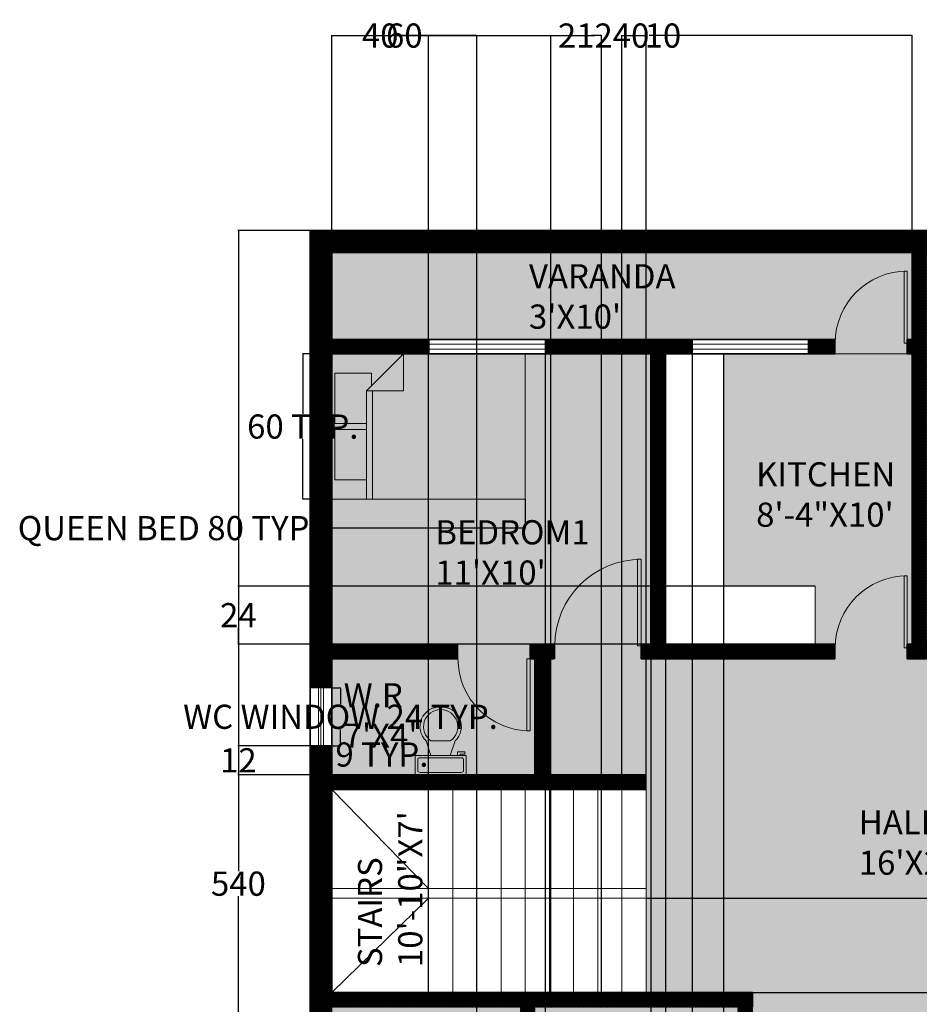
# Model space of a CAD drawing. Units: inches. Extents: x -89252 to 1164, y -183799 to 823.
# Tile 3 of 4: x 600 to 972, y 416 to 823. Entities that reach past the tile are written whole.
import ezdxf

# ---------------------------------------------------------------- set-up
doc = ezdxf.new("R2010")
doc.units = ezdxf.units.IN
doc.header["$MEASUREMENT"] = 0
for name, color, linetype, lineweight in [('A-ANNO-DIMS', 2, 'Continuous', 18), ('A-AREA-IDEN', 7, 'Continuous', 25), ('A-FLOR-CASE', 8, 'Continuous', 18), ('A-FLOR-STRS', 7, 'Continuous', 18), ('A-GLAZ', 4, 'Continuous', 18), ('A-WALL', 7, 'Continuous', 35), ('BED', 7, 'Continuous', 18), ('DOOR', 7, 'Continuous', 18), ('TOILET', 7, 'Continuous', 18)]:
    doc.layers.add(name, color=color, linetype=linetype, lineweight=lineweight)
doc.layers.add('A-FLOR-PATT', color=252, linetype='Continuous', lineweight=13, true_color=0x939598)
doc.layers.add('A-WALL-PATT', color=18, linetype='Continuous', lineweight=13, true_color=0x000000)
doc.styles.get("Standard").update_dxf_attribs({"font": 'arial.ttf'})
doc.dimstyles.get("Standard").update_dxf_attribs({"dimtxt": 10, "dimasz": 0.18, "dimexe": 0.18, "dimexo": 0.0625, "dimgap": 0.09, "dimtad": 0, "dimtih": 1, "dimtoh": 1, "dimdec": 0, "dimzin": 0, "dimdsep": 46, "dimlunit": 3, "dimtxsty": 'Standard', "dimcen": 0.09, "dimadec": 0, "dimazin": 0, "dimtfac": 1, "dimtdec": 0, "dimtofl": 0, "dimtmove": 0, "dimatfit": 3, "dimfxl": 1, "dimtolj": 1, "dimtzin": 0, "dimarcsym": 0})

# ---------------------------------------------------------------- blocks, each defined once
blk = doc.blocks.new('*U3')
for p, q in [((0, 0), (0, -6)), ((40, 0), (40, -6))]:
    blk.add_line(p, q)
blk.add_lwpolyline([(0, 0), (0, 40), (1.75, 40), (1.75, 0)], close=True)
blk.add_arc((0, 0), 40, 0, 90)
blk = doc.blocks.new('*U4')
for p, q in [((0, 0), (0, 6)), ((40, 0), (40, 6))]:
    blk.add_line(p, q)
blk.add_lwpolyline([(0, 0), (0, -40), (1.75, -40), (1.75, 0)], close=True)
blk.add_arc((0, 0), 40, 270, 0)
blk = doc.blocks.new('Bed - Queen')
for p, q in [((0, -80.00003), (0, 0)), ((0, 0), (59.99999, 0)), ((59.99999, 0), (59.99999, -80.00003)), ((7.99999, -1.2), (28.79998, -1.2)), ((7.99999, -14.4), (7.99999, -1.2)), ((28.79998, -1.2), (28.79998, -14.4)), ((31.19999, -1.2), (51.99999, -1.2)), ((31.19999, -14.4), (31.19999, -1.2)), ((51.99999, -1.2), (51.99999, -16.4)), ((0, -14.4), (44.8, -14.4)), ((59.99999, -29.6), (44.8, -14.4)), ((44.8, -14.4), (44.8, -29.6)), ((44.8, -16.8), (0, -16.8)), ((51.99999, -16.4), (46.79936, -16.4)), ((44.8, -29.6), (59.99999, -29.6)), ((59.99999, -80.00003), (0, -80.00003))]:
    blk.add_line(p, q)
blk = doc.blocks.new('*U12')
for p, q in [((9.5, -6), (9.5, -2)), ((-8, -8.5), (-8, -8)), ((-7, -8), (-7, -9.5)), ((-4, -8), (-6, -14)), ((4, -8), (6, -14)), ((-10, -8.5), (-8, -8.5)), ((-10, -9.5), (-10, -8.5)), ((-7, -9.5), (-10, -9.5)), ((4, -14), (-4, -14))]:
    blk.add_line(p, q)
blk.add_lwpolyline([(10.5, -8), (10.5, 0), (-10.5, 0), (-10.5, -8)], close=True)
for points in [[(-9.5, -2), (-9.5, -6)], [(8.5, -1), (-8.5, -1)], [(-8.5, -7), (8.5, -7)]]:
    blk.add_lwpolyline(points)
for centre, radius, start, end in [((-8.625, -1.875), 0.8839, 81.8699, 188.1301), ((8.625, -1.875), 0.8839, 351.8699, 98.1301), ((-8.625, -6.125), 0.8839, 171.869898, 278.1301), ((8.625, -6.125), 0.8839, 261.8699, 8.1301), ((-0.4772, -19.9188), 8.0953, 133.01722, 273.38), ((0.0374, -19.8731), 7.127, 124.50543, 269.7), ((-0.0373, -19.8731), 7.127, 270.3, 55.4946), ((0.4773, -19.9188), 8.0953, 266.62, 46.9828)]:
    blk.add_arc(centre, radius, start, end)
blk = doc.blocks.new('WIN-24IN-9IN-WALL')
for p, q in [((9, 24), (0, 24)), ((3.5, 0), (3.5, 24)), ((4.5, 0), (4.5, 24)), ((5.5, 0), (5.5, 24)), ((9, 0), (0, 0))]:
    blk.add_line(p, q)
blk = doc.blocks.new('WIN-48IN-6IN-WALL')
for p, q in [((0, 0), (0, 6)), ((48, 0), (48, 6)), ((0, 4), (48, 4)), ((0, 2), (48, 2))]:
    blk.add_line(p, q)
blk = doc.blocks.new('*D18')
at = {"layer": 'A-ANNO-DIMS', "color": 0, "lineweight": -2, "transparency": 16777216}
for p, q in [((729.36, 624.33), (729.36, 612.21)), ((809.36, 624.33), (809.36, 612.21)), ((729.36, 612.39), (729.18, 612.39)), ((809.18, 612.39), (729.54, 612.39))]:
    blk.add_line(p, q, dxfattribs=at)
at = {"layer": 'A-ANNO-DIMS', "color": 0, "transparency": 16777216}
for points in [[(729.54, 612.42), (729.54, 612.36), (729.36, 612.39)], [(809.18, 612.42), (809.18, 612.36), (809.36, 612.39)]]:
    blk.add_solid(points, dxfattribs=at)
at = {"layer": 'Defpoints', "color": 0, "transparency": 16777216}
for p in [(729.36, 624.39), (809.36, 624.39), (729.36, 612.39)]:
    blk.add_point(p, dxfattribs=at)
at = {"layer": 'A-ANNO-DIMS', "color": 0, "transparency": 16777216, "insert": (661.68, 612.39), "char_height": 10, "attachment_point": 5}
blk.add_mtext('\\A1;QUEEN BED 80 TYP.', dxfattribs=at)
blk = doc.blocks.new('*D19')
at = {"layer": 'A-ANNO-DIMS', "color": 0, "lineweight": -2, "transparency": 16777216}
for p, q in [((729.3, 684.39), (717.18, 684.39)), ((717.36, 684.21), (717.36, 659.59)), ((717.36, 624.57), (717.36, 649.19)), ((729.3, 624.39), (717.18, 624.39))]:
    blk.add_line(p, q, dxfattribs=at)
at = {"layer": 'A-ANNO-DIMS', "color": 0, "transparency": 16777216}
for points in [[(717.33, 684.21), (717.39, 684.21), (717.36, 684.39)], [(717.33, 624.57), (717.39, 624.57), (717.36, 624.39)]]:
    blk.add_solid(points, dxfattribs=at)
at = {"layer": 'Defpoints', "color": 0, "transparency": 16777216}
for p in [(717.36, 684.39), (729.36, 684.39), (729.36, 624.39)]:
    blk.add_point(p, dxfattribs=at)
at = {"layer": 'A-ANNO-DIMS', "color": 0, "transparency": 16777216, "insert": (717.36, 654.39), "char_height": 10, "attachment_point": 5}
blk.add_mtext('\\A1;60 TYP.', dxfattribs=at)
blk = doc.blocks.new('*D20')
at = {"layer": 'A-ANNO-DIMS', "color": 0, "lineweight": -2, "transparency": 16777216}
for p, q in [((729.43, 546.39), (733.14, 546.39)), ((732.96, 546.21), (732.96, 539.65)), ((732.96, 522.57), (732.96, 529.13)), ((729.43, 522.39), (733.14, 522.39))]:
    blk.add_line(p, q, dxfattribs=at)
at = {"layer": 'A-ANNO-DIMS', "color": 0, "transparency": 16777216}
for points in [[(732.93, 546.21), (732.99, 546.21), (732.96, 546.39)], [(732.93, 522.57), (732.99, 522.57), (732.96, 522.39)]]:
    blk.add_solid(points, dxfattribs=at)
at = {"layer": 'Defpoints', "color": 0, "transparency": 16777216}
for p in [(729.36, 546.39), (732.96, 546.39), (729.36, 522.39)]:
    blk.add_point(p, dxfattribs=at)
at = {"layer": 'A-ANNO-DIMS', "color": 0, "transparency": 16777216, "insert": (732.96, 534.39), "char_height": 10, "attachment_point": 5}
blk.add_mtext('\\A1;WC WINDOW 24 TYP.', dxfattribs=at)
blk = doc.blocks.new('*D21')
at = {"layer": 'A-ANNO-DIMS', "color": 0, "lineweight": -2, "transparency": 16777216}
for p, q in [((720.36, 522.33), (720.36, 518.61)), ((729.36, 522.33), (729.36, 518.61)), ((720.54, 518.79), (729.18, 518.79)), ((729.36, 518.79), (729.54, 518.79))]:
    blk.add_line(p, q, dxfattribs=at)
at = {"layer": 'A-ANNO-DIMS', "color": 0, "transparency": 16777216}
for points in [[(720.54, 518.82), (720.54, 518.76), (720.36, 518.79)], [(729.18, 518.82), (729.18, 518.76), (729.36, 518.79)]]:
    blk.add_solid(points, dxfattribs=at)
at = {"layer": 'Defpoints', "color": 0, "transparency": 16777216}
for p in [(720.36, 522.39), (729.36, 522.39), (729.36, 518.79)]:
    blk.add_point(p, dxfattribs=at)
at = {"layer": 'A-ANNO-DIMS', "color": 0, "transparency": 16777216, "insert": (750.09, 518.79), "char_height": 10, "attachment_point": 5}
blk.add_mtext('\\A1;9 TYP.', dxfattribs=at)
blk = doc.blocks.new('*D31')
at = {"layer": 'A-ANNO-DIMS', "color": 0, "lineweight": -2, "transparency": 16777216}
for p, q in [((720.3, 735.39), (690.53, 735.39)), ((690.71, 735.21), (690.71, 470.59)), ((690.71, 195.57), (690.71, 460.19)), ((720.3, 195.39), (690.53, 195.39))]:
    blk.add_line(p, q, dxfattribs=at)
at = {"layer": 'A-ANNO-DIMS', "color": 0, "transparency": 16777216}
for points in [[(690.68, 735.21), (690.74, 735.21), (690.71, 735.39)], [(690.68, 195.57), (690.74, 195.57), (690.71, 195.39)]]:
    blk.add_solid(points, dxfattribs=at)
at = {"layer": 'Defpoints', "color": 0, "transparency": 16777216}
for p in [(690.71, 735.39), (720.36, 735.39), (720.36, 195.39)]:
    blk.add_point(p, dxfattribs=at)
at = {"layer": 'A-ANNO-DIMS', "color": 0, "transparency": 16777216, "insert": (690.71, 465.39), "char_height": 10, "attachment_point": 5}
blk.add_mtext('\\A1;540', dxfattribs=at)
blk = doc.blocks.new('*D33')
at = {"layer": 'A-ANNO-DIMS', "color": 0, "lineweight": -2, "transparency": 16777216}
for p, q in [((729.36, 726.45), (729.36, 816.22)), ((729.54, 816.04), (838.16, 816.04)), ((969.18, 816.04), (860.57, 816.04)), ((969.36, 726.45), (969.36, 816.22))]:
    blk.add_line(p, q, dxfattribs=at)
at = {"layer": 'A-ANNO-DIMS', "color": 0, "transparency": 16777216}
for points in [[(729.54, 816.07), (729.54, 816.01), (729.36, 816.04)], [(969.18, 816.07), (969.18, 816.01), (969.36, 816.04)]]:
    blk.add_solid(points, dxfattribs=at)
at = {"layer": 'Defpoints', "color": 0, "transparency": 16777216}
for p in [(969.36, 816.04), (729.36, 726.39), (969.36, 726.39)]:
    blk.add_point(p, dxfattribs=at)
at = {"layer": 'A-ANNO-DIMS', "color": 0, "transparency": 16777216, "insert": (849.36, 816.04), "char_height": 10, "attachment_point": 5}
blk.add_mtext('\\A1;240', dxfattribs=at)
blk = doc.blocks.new('*D41')
at = {"layer": 'A-ANNO-DIMS', "color": 0, "lineweight": -2, "transparency": 16777216}
for p, q in [((729.36, 240.45), (729.36, 816.22)), ((729.54, 816.04), (752.1, 816.04)), ((789.18, 816.04), (766.63, 816.04)), ((789.36, 240.45), (789.36, 816.22))]:
    blk.add_line(p, q, dxfattribs=at)
at = {"layer": 'A-ANNO-DIMS', "color": 0, "transparency": 16777216}
for points in [[(729.54, 816.07), (729.54, 816.01), (729.36, 816.04)], [(789.18, 816.07), (789.18, 816.01), (789.36, 816.04)]]:
    blk.add_solid(points, dxfattribs=at)
at = {"layer": 'Defpoints', "color": 0, "transparency": 16777216}
for p in [(789.36, 816.04), (729.36, 240.39), (789.36, 240.39)]:
    blk.add_point(p, dxfattribs=at)
at = {"layer": 'A-ANNO-DIMS', "color": 0, "transparency": 16777216, "insert": (759.36, 816.04), "char_height": 10, "attachment_point": 5}
blk.add_mtext('\\A1;60', dxfattribs=at)
blk = doc.blocks.new('*D43')
at = {"layer": 'A-ANNO-DIMS', "color": 0, "lineweight": -2, "transparency": 16777216}
for p, q in [((849.36, 504.45), (849.36, 816.22)), ((849.54, 816.04), (859.18, 816.04)), ((859.36, 504.45), (859.36, 816.22)), ((859.36, 816.04), (859.54, 816.04))]:
    blk.add_line(p, q, dxfattribs=at)
at = {"layer": 'A-ANNO-DIMS', "color": 0, "transparency": 16777216}
for points in [[(849.54, 816.07), (849.54, 816.01), (849.36, 816.04)], [(859.18, 816.07), (859.18, 816.01), (859.36, 816.04)]]:
    blk.add_solid(points, dxfattribs=at)
at = {"layer": 'Defpoints', "color": 0, "transparency": 16777216}
for p in [(859.36, 816.04), (849.36, 504.39), (859.36, 504.39)]:
    blk.add_point(p, dxfattribs=at)
at = {"layer": 'A-ANNO-DIMS', "color": 0, "transparency": 16777216, "insert": (866.31, 816.04), "char_height": 10, "attachment_point": 5}
blk.add_mtext('\\A1;10', dxfattribs=at)
blk = doc.blocks.new('*D44')
at = {"layer": 'A-ANNO-DIMS', "color": 0, "lineweight": -2, "transparency": 16777216}
for p, q in [((867.36, 684.33), (867.36, 165.56)), ((891.36, 684.33), (891.36, 165.56)), ((867.54, 165.74), (872.05, 165.74)), ((891.18, 165.74), (886.68, 165.74))]:
    blk.add_line(p, q, dxfattribs=at)
at = {"layer": 'A-ANNO-DIMS', "color": 0, "transparency": 16777216}
for points in [[(867.54, 165.77), (867.54, 165.71), (867.36, 165.74)], [(891.18, 165.77), (891.18, 165.71), (891.36, 165.74)]]:
    blk.add_solid(points, dxfattribs=at)
at = {"layer": 'Defpoints', "color": 0, "transparency": 16777216}
for p in [(867.36, 684.39), (891.36, 684.39), (891.36, 165.74)]:
    blk.add_point(p, dxfattribs=at)
at = {"layer": 'A-ANNO-DIMS', "color": 0, "transparency": 16777216, "insert": (879.36, 165.74), "char_height": 10, "attachment_point": 5}
blk.add_mtext('\\A1;24', dxfattribs=at)
blk = doc.blocks.new('*D45')
at = {"layer": 'A-ANNO-DIMS', "color": 0, "lineweight": -2, "transparency": 16777216}
for p, q in [((929.24, 588.39), (690.53, 588.39)), ((690.71, 588.21), (690.71, 581.5)), ((690.71, 564.57), (690.71, 571.28)), ((929.24, 564.39), (690.53, 564.39))]:
    blk.add_line(p, q, dxfattribs=at)
at = {"layer": 'A-ANNO-DIMS', "color": 0, "transparency": 16777216}
for points in [[(690.68, 588.21), (690.74, 588.21), (690.71, 588.39)], [(690.68, 564.57), (690.74, 564.57), (690.71, 564.39)]]:
    blk.add_solid(points, dxfattribs=at)
at = {"layer": 'Defpoints', "color": 0, "transparency": 16777216}
for p in [(690.71, 588.39), (929.31, 588.39), (929.31, 564.39)]:
    blk.add_point(p, dxfattribs=at)
at = {"layer": 'A-ANNO-DIMS', "color": 0, "transparency": 16777216, "insert": (690.71, 576.39), "char_height": 10, "attachment_point": 5}
blk.add_mtext('\\A1;24', dxfattribs=at)
blk = doc.blocks.new('*D47')
at = {"layer": 'A-ANNO-DIMS', "color": 0, "lineweight": -2, "transparency": 16777216}
for p, q in [((817.67, 690.33), (817.67, 165.56)), ((878.36, 690.33), (878.36, 165.56)), ((817.85, 165.74), (831.02, 165.74)), ((878.18, 165.74), (865.02, 165.74))]:
    blk.add_line(p, q, dxfattribs=at)
at = {"layer": 'A-ANNO-DIMS', "color": 0, "transparency": 16777216}
for points in [[(817.85, 165.77), (817.85, 165.71), (817.67, 165.74)], [(878.18, 165.77), (878.18, 165.71), (878.36, 165.74)]]:
    blk.add_solid(points, dxfattribs=at)
at = {"layer": 'Defpoints', "color": 0, "transparency": 16777216}
for p in [(817.67, 690.39), (878.36, 690.39), (878.36, 165.74)]:
    blk.add_point(p, dxfattribs=at)
at = {"layer": 'A-ANNO-DIMS', "color": 0, "transparency": 16777216, "insert": (848.02, 165.74), "char_height": 10, "attachment_point": 5}
blk.add_mtext('\\A1;60.69', dxfattribs=at)
blk = doc.blocks.new('*D48')
at = {"layer": 'A-ANNO-DIMS', "color": 0, "lineweight": -2, "transparency": 16777216}
for p, q in [((817.67, 684.33), (817.67, 165.56)), ((861.36, 684.33), (861.36, 165.56)), ((817.85, 165.74), (822.34, 165.74)), ((861.18, 165.74), (856.69, 165.74))]:
    blk.add_line(p, q, dxfattribs=at)
at = {"layer": 'A-ANNO-DIMS', "color": 0, "transparency": 16777216}
for points in [[(817.85, 165.77), (817.85, 165.71), (817.67, 165.74)], [(861.18, 165.77), (861.18, 165.71), (861.36, 165.74)]]:
    blk.add_solid(points, dxfattribs=at)
at = {"layer": 'Defpoints', "color": 0, "transparency": 16777216}
for p in [(817.67, 684.39), (861.36, 684.39), (861.36, 165.74)]:
    blk.add_point(p, dxfattribs=at)
at = {"layer": 'A-ANNO-DIMS', "color": 0, "transparency": 16777216, "insert": (839.52, 165.74), "char_height": 10, "attachment_point": 5}
blk.add_mtext('\\A1;43.69', dxfattribs=at)
blk = doc.blocks.new('*D50')
at = {"layer": 'A-ANNO-DIMS', "color": 0, "lineweight": -2, "transparency": 16777216}
for p, q in [((729.3, 522.39), (690.53, 522.39)), ((690.71, 522.21), (690.71, 521.5)), ((729.3, 510.39), (690.53, 510.39)), ((690.71, 510.57), (690.71, 511.28))]:
    blk.add_line(p, q, dxfattribs=at)
at = {"layer": 'A-ANNO-DIMS', "color": 0, "transparency": 16777216}
for points in [[(690.68, 522.21), (690.74, 522.21), (690.71, 522.39)], [(690.68, 510.57), (690.74, 510.57), (690.71, 510.39)]]:
    blk.add_solid(points, dxfattribs=at)
at = {"layer": 'Defpoints', "color": 0, "transparency": 16777216}
for p in [(729.36, 522.39), (690.71, 510.39), (729.36, 510.39)]:
    blk.add_point(p, dxfattribs=at)
at = {"layer": 'A-ANNO-DIMS', "color": 0, "transparency": 16777216, "insert": (690.71, 516.39), "char_height": 10, "attachment_point": 5}
blk.add_mtext('\\A1;12', dxfattribs=at)
blk = doc.blocks.new('*D51')
at = {"layer": 'A-ANNO-DIMS', "color": 0, "lineweight": -2, "transparency": 16777216}
for p, q in [((729.36, 420.45), (729.36, 816.22)), ((729.54, 816.04), (741.93, 816.04)), ((769.18, 816.04), (756.8, 816.04)), ((769.36, 420.45), (769.36, 816.22))]:
    blk.add_line(p, q, dxfattribs=at)
at = {"layer": 'A-ANNO-DIMS', "color": 0, "transparency": 16777216}
for points in [[(729.54, 816.07), (729.54, 816.01), (729.36, 816.04)], [(769.18, 816.07), (769.18, 816.01), (769.36, 816.04)]]:
    blk.add_solid(points, dxfattribs=at)
at = {"layer": 'Defpoints', "color": 0, "transparency": 16777216}
for p in [(729.36, 816.04), (729.36, 420.39), (769.36, 420.39)]:
    blk.add_point(p, dxfattribs=at)
at = {"layer": 'A-ANNO-DIMS', "color": 0, "transparency": 16777216, "insert": (749.36, 816.04), "char_height": 10, "attachment_point": 5}
blk.add_mtext('\\A1;40', dxfattribs=at)
blk = doc.blocks.new('*D52')
at = {"layer": 'A-ANNO-DIMS', "color": 0, "lineweight": -2, "transparency": 16777216}
for p, q in [((859.43, 459.39), (1134.19, 459.39)), ((1134.01, 459.21), (1134.01, 445.09)), ((1134.01, 420.57), (1134.01, 434.69)), ((859.43, 420.39), (1134.19, 420.39))]:
    blk.add_line(p, q, dxfattribs=at)
at = {"layer": 'A-ANNO-DIMS', "color": 0, "transparency": 16777216}
for points in [[(1133.98, 459.21), (1134.04, 459.21), (1134.01, 459.39)], [(1133.98, 420.57), (1134.04, 420.57), (1134.01, 420.39)]]:
    blk.add_solid(points, dxfattribs=at)
at = {"layer": 'Defpoints', "color": 0, "transparency": 16777216}
for p in [(859.36, 459.39), (1134.01, 459.39), (859.36, 420.39)]:
    blk.add_point(p, dxfattribs=at)
at = {"layer": 'A-ANNO-DIMS', "color": 0, "transparency": 16777216, "insert": (1134.01, 439.89), "char_height": 10, "attachment_point": 5}
blk.add_mtext('\\A1;39', dxfattribs=at)
blk = doc.blocks.new('*D53')
at = {"layer": 'A-ANNO-DIMS', "color": 0, "lineweight": -2, "transparency": 16777216}
for p, q in [((819.96, 414.26), (819.96, 816.22)), ((820.14, 816.04), (824.09, 816.04)), ((840.78, 816.04), (836.83, 816.04)), ((840.96, 414.26), (840.96, 816.22))]:
    blk.add_line(p, q, dxfattribs=at)
at = {"layer": 'A-ANNO-DIMS', "color": 0, "transparency": 16777216}
for points in [[(820.14, 816.07), (820.14, 816.01), (819.96, 816.04)], [(840.78, 816.07), (840.78, 816.01), (840.96, 816.04)]]:
    blk.add_solid(points, dxfattribs=at)
at = {"layer": 'Defpoints', "color": 0, "transparency": 16777216}
for p in [(840.96, 816.04), (819.96, 414.2), (840.96, 414.2)]:
    blk.add_point(p, dxfattribs=at)
at = {"layer": 'A-ANNO-DIMS', "color": 0, "transparency": 16777216, "insert": (830.46, 816.04), "char_height": 10, "attachment_point": 5}
blk.add_mtext('\\A1;21', dxfattribs=at)

msp = doc.modelspace()

# ---------------------------------------------------------------- hatches: boundary and pattern name
at = {"layer": 'A-FLOR-PATT'}
h = msp.add_hatch(color=256, dxfattribs=at)
h.dxf.hatch_style = 1
h.paths.add_polyline_path([(1095.364, 558.3893), (1013.364, 558.3893), (1013.364, 564.3893), (1095.364, 564.3893), (1095.364, 672.3893), (1093.364, 672.3893), (1063.364, 672.3893), (1005.364, 672.3893), (1005.364, 726.3893), (975.364, 726.3893), (975.364, 690.3893), (975.364, 564.3893), (977.364, 564.3893), (977.364, 558.3893), (975.364, 558.3893), (969.364, 558.3893), (967.364, 558.3893), (967.364, 564.3893), (969.364, 564.3893), (969.364, 684.3893), (967.364, 684.3893), (937.364, 684.3893), (891.364, 684.3893), (891.364, 588.3893), (929.3053, 588.3893), (929.3053, 564.3893), (937.364, 564.3893), (937.364, 558.3893), (857.364, 558.3893), (857.364, 564.3893), (861.364, 564.3893), (861.364, 684.3893), (729.364, 684.3893), (729.364, 564.3893), (781.364, 564.3893), (781.364, 558.3893), (729.364, 558.3893), (729.364, 510.3893), (813.364, 510.3893), (813.364, 558.3893), (811.364, 558.3893), (811.364, 564.3893), (813.364, 564.3893), (819.364, 564.3893), (821.364, 564.3893), (821.364, 558.3893), (819.364, 558.3893), (819.364, 510.3893), (859.364, 510.3893), (859.364, 420.3893), (903.364, 420.3893), (903.364, 414.3893), (903.364, 412.3893), (897.364, 412.3893), (897.364, 414.3893), (813.364, 414.3893), (813.364, 366.3893), (897.364, 366.3893), (897.364, 382.3893), (903.364, 382.3893), (903.364, 360.3893), (903.364, 358.3893), (897.364, 358.3893), (897.364, 360.3893), (807.364, 360.3893), (805.364, 360.3893), (805.364, 366.3893), (807.364, 366.3893), (807.364, 414.3893), (729.364, 414.3893), (729.364, 366.3893), (775.364, 366.3893), (775.364, 360.3893), (729.364, 360.3893), (729.364, 240.3893), (897.364, 240.3893), (897.364, 318.3893), (1021.364, 318.3893), (1021.364, 312.3893), (1071.364, 312.3893), (1071.364, 318.3893), (1095.364, 318.3893)])
h.paths.add_polyline_path([(1095.364, 726.3893), (1011.364, 726.3893), (1011.364, 678.3893), (1063.364, 678.3893), (1063.364, 672.3893), (1093.364, 672.3893), (1093.364, 678.3893), (1095.364, 678.3893)])
h.paths.add_polyline_path([(969.364, 726.3893), (729.364, 726.3893), (729.364, 690.3893), (937.364, 690.3893), (937.364, 684.3893), (967.364, 684.3893), (967.364, 690.3893), (969.364, 690.3893)])
at = {"layer": 'A-WALL-PATT'}
h = msp.add_hatch(dxfattribs=at)
h.set_pattern_fill('ANSI31', color=256)
h.paths.add_polyline_path([(867.364, 684.3893), (878.364, 684.3893), (878.364, 690.3893), (817.6735, 690.3893), (817.6735, 684.3893), (861.364, 684.3893), (861.364, 564.3893), (857.364, 564.3893), (857.364, 558.3893), (937.364, 558.3893), (937.364, 564.3893), (867.364, 564.3893)], flags=17)
h.paths.add_polyline_path([(1041.364, 735.3893), (720.364, 735.3893), (720.364, 546.3893), (729.364, 546.3893), (729.364, 558.3893), (781.364, 558.3893), (781.364, 564.3893), (729.364, 564.3893), (729.364, 684.3893), (769.6735, 684.3893), (769.6735, 690.3893), (729.364, 690.3893), (729.364, 726.3893), (969.364, 726.3893), (969.364, 690.3893), (967.364, 690.3893), (967.364, 684.3893), (969.364, 684.3893), (969.364, 564.3893), (967.364, 564.3893), (967.364, 558.3893), (969.364, 558.3893), (975.364, 558.3893), (977.364, 558.3893), (977.364, 564.3893), (975.364, 564.3893), (975.364, 690.3893), (975.364, 726.3893), (1005.364, 726.3893), (1005.364, 672.3893), (1063.364, 672.3893), (1063.364, 678.3893), (1011.364, 678.3893), (1011.364, 726.3893), (1041.364, 726.3893)])
h.paths.add_polyline_path([(1104.364, 735.3893), (1065.364, 735.3893), (1065.364, 726.3893), (1095.364, 726.3893), (1095.364, 678.3893), (1093.364, 678.3893), (1093.364, 672.3893), (1095.364, 672.3893), (1095.364, 642.3893), (1104.364, 642.3893)])
h.paths.add_polyline_path([(1104.364, 594.3893), (1095.364, 594.3893), (1095.364, 564.3893), (1013.364, 564.3893), (1013.364, 558.3893), (1095.364, 558.3893), (1095.364, 515.2697), (1104.364, 515.2697)])
h.paths.add_polyline_path([(1104.364, 467.2697), (1095.364, 467.2697), (1095.364, 419.2348), (1104.364, 419.2348)])
h.paths.add_polyline_path([(1104.364, 371.2348), (1095.364, 371.2348), (1095.364, 312.3893), (1104.364, 312.3893)], flags=17)
h.paths.add_polyline_path([(1095.364, 318.3893), (1071.364, 318.3893), (1071.364, 312.3893), (1095.364, 312.3893)], flags=17)
h.paths.add_polyline_path([(1021.364, 318.3893), (897.364, 318.3893), (897.364, 240.3893), (837.364, 240.3893), (837.364, 234.3893), (903.364, 234.3893), (903.364, 312.3893), (1021.364, 312.3893)], flags=17)
h.paths.add_polyline_path([(903.364, 382.3893), (897.364, 382.3893), (897.364, 366.3893), (813.364, 366.3893), (813.364, 414.3893), (897.364, 414.3893), (897.364, 412.3893), (903.364, 412.3893), (903.364, 414.3893), (903.364, 420.3893), (729.364, 420.3893), (729.364, 504.3893), (859.364, 504.3893), (859.364, 510.3893), (819.364, 510.3893), (819.364, 558.3893), (821.364, 558.3893), (821.364, 564.3893), (819.364, 564.3893), (813.364, 564.3893), (811.364, 564.3893), (811.364, 558.3893), (813.364, 558.3893), (813.364, 510.3893), (729.364, 510.3893), (729.364, 522.3893), (720.364, 522.3893), (720.364, 400.5349), (729.364, 400.5349), (729.364, 414.3893), (807.364, 414.3893), (807.364, 366.3893), (805.364, 366.3893), (805.364, 360.3893), (807.364, 360.3893), (897.364, 360.3893), (897.364, 358.3893), (903.364, 358.3893), (903.364, 360.3893)])
h.paths.add_polyline_path([(775.364, 366.3893), (729.364, 366.3893), (729.364, 376.5349), (720.364, 376.5349), (720.364, 195.3893), (1104.364, 195.3893), (1104.364, 204.3893), (729.364, 204.3893), (729.364, 234.3893), (789.364, 234.3893), (789.364, 240.3893), (729.364, 240.3893), (729.364, 360.3893), (775.364, 360.3893)])
h.paths.add_polyline_path([(937.364, 690.3893), (926.364, 690.3893), (926.364, 684.3893), (937.364, 684.3893)], flags=17)

# ---------------------------------------------------------------- linework, layer by layer
at = {"layer": 'A-FLOR-CASE'}
for p, q in [((891.364, 684.3893), (891.364, 588.3893)), ((929.3053, 588.3893), (891.364, 588.3893)), ((929.3053, 564.3893), (929.3053, 588.3893))]:
    msp.add_line(p, q, dxfattribs=at)
at = {"layer": 'A-FLOR-STRS'}
for p, q in [((859.364, 510.3893), (859.364, 420.3893)), ((769.364, 463.3893), (729.364, 504.3893)), ((769.364, 504.3893), (769.364, 420.3893)), ((779.364, 504.3893), (779.364, 420.3893)), ((789.364, 504.3893), (789.364, 420.3893)), ((799.364, 504.3893), (799.364, 420.3893)), ((809.364, 504.3893), (809.364, 420.3893)), ((819.364, 504.3893), (819.364, 420.3893)), ((829.364, 504.3893), (829.364, 420.3893)), ((839.364, 504.3893), (839.364, 420.3893)), ((849.364, 504.3893), (849.364, 420.3893)), ((859.364, 463.3893), (729.364, 463.3893)), ((859.364, 459.3893), (729.364, 459.3893)), ((769.364, 459.3893), (729.364, 420.3893))]:
    msp.add_line(p, q, dxfattribs=at)
at = {"layer": 'A-WALL'}
for p, q in [((1104.364, 735.3893), (720.364, 735.3893)), ((720.364, 735.3893), (720.364, 195.3893)), ((729.364, 726.3893), (729.364, 690.3893)), ((969.364, 726.3893), (729.364, 726.3893)), ((969.364, 690.3893), (969.364, 726.3893)), ((937.364, 690.3893), (729.364, 690.3893)), ((937.364, 684.3893), (937.364, 690.3893)), ((969.364, 690.3893), (967.364, 690.3893)), ((967.364, 690.3893), (967.364, 684.3893)), ((729.364, 684.3893), (729.364, 564.3893)), ((861.364, 684.3893), (729.364, 684.3893)), ((861.364, 684.3893), (861.364, 564.3893)), ((867.364, 684.3893), (867.364, 564.3893)), ((937.364, 684.3893), (867.364, 684.3893)), ((867.364, 684.3893), (937.364, 684.3893)), ((967.364, 684.3893), (969.364, 684.3893)), ((969.364, 564.3893), (969.364, 684.3893)), ((781.364, 564.3893), (729.364, 564.3893)), ((781.364, 564.3893), (781.364, 558.3893)), ((811.364, 558.3893), (811.364, 564.3893)), ((811.364, 564.3893), (813.364, 564.3893)), ((819.364, 564.3893), (813.364, 564.3893)), ((821.364, 564.3893), (819.364, 564.3893)), ((821.364, 558.3893), (821.364, 564.3893)), ((857.364, 564.3893), (857.364, 558.3893)), ((861.364, 564.3893), (857.364, 564.3893)), ((937.364, 564.3893), (867.364, 564.3893)), ((937.364, 558.3893), (937.364, 564.3893)), ((937.364, 558.3893), (937.364, 564.3893)), ((969.364, 564.3893), (967.364, 564.3893)), ((967.364, 564.3893), (967.364, 558.3893)), ((781.364, 558.3893), (729.364, 558.3893)), ((729.364, 510.3893), (729.364, 558.3893)), ((729.364, 558.3893), (729.364, 510.3893)), ((813.364, 558.3893), (811.364, 558.3893)), ((813.364, 558.3893), (813.364, 510.3893)), ((819.364, 558.3893), (819.364, 510.3893)), ((819.364, 558.3893), (821.364, 558.3893)), ((937.364, 558.3893), (857.364, 558.3893)), ((967.364, 558.3893), (969.364, 558.3893)), ((975.364, 558.3893), (969.364, 558.3893)), ((813.364, 510.3893), (729.364, 510.3893)), ((859.364, 510.3893), (819.364, 510.3893)), ((859.364, 504.3893), (729.364, 504.3893)), ((729.364, 504.3893), (729.364, 420.3893)), ((903.364, 420.3893), (729.364, 420.3893)), ((903.364, 420.3893), (903.364, 414.3893))]:
    msp.add_line(p, q, dxfattribs=at)
at = {"layer": 'DOOR'}
msp.add_line((937.364, 684.3893), (967.364, 684.3893), dxfattribs=at)

# ---------------------------------------------------------------- block references
at = {"layer": 'A-GLAZ'}
for name, p in [('WIN-48IN-6IN-WALL', (769.6734, 684.389)), ('WIN-48IN-6IN-WALL', (878.364, 684.389)), ('WIN-24IN-9IN-WALL', (720.364, 522.389))]:
    msp.add_blockref(name, p, dxfattribs=at)
at = {"layer": 'BED', "rotation": 90}
msp.add_blockref('Bed - Queen', (729.364, 624.3893), dxfattribs=at)
at = {"layer": 'DOOR'}
for name, p, xscale, yscale, zscale in [('*U3', (967.364, 688.863), -0.7456098286251903, 0.7456098286251903, 0.7456098286251903), ('*U3', (857.364, 563.7517), -0.8937210586509982, 0.8937210586509982, 0.8937210586509982), ('*U3', (967.364, 562.863), -0.7456098286251903, 0.7456098286251903, 0.7456098286251903), ('*U4', (811.364, 558.3893), -0.7456098286251903, 0.7456098286251903, 0.7456098286251903)]:
    msp.add_blockref(name, p, dxfattribs=dict(at, xscale=xscale, yscale=yscale, zscale=zscale))
at = {"layer": 'TOILET', "rotation": 180}
msp.add_blockref('*U12', (774.3827, 510.3893), dxfattribs=at)

# ---------------------------------------------------------------- texts
at = {"layer": 'A-AREA-IDEN', "char_height": 10, "attachment_point": 1}
for s, insert in [("VARANDA\\P3'X10'", (810.9079, 721.5138)), ('KITCHEN\\P8\'-4"X10\'', (904.8759, 639.6262)), ("BEDROM1\\P11'X10'", (772.1588, 615.6697)), ("W.R\\P7'X4'", (734.2797, 548.2568)), ("HALL\\P16'X20'", (947.3283, 495.7486))]:
    msp.add_mtext_dynamic_manual_height_columns(s, width=99.889598, gutter_width=1, heights=[0], dxfattribs=dict(at, insert=insert))
at = {"layer": 'A-AREA-IDEN', "insert": (740.1502, 430.9059), "char_height": 10, "attachment_point": 1, "rotation": 90}
msp.add_mtext_dynamic_manual_height_columns('\\pxt1;STAIRS\\P10\'-10"X7\'', width=99.889598, gutter_width=1, heights=[0], dxfattribs=at)

# ---------------------------------------------------------------- dimensions: what is measured, and where the dimension line sits
at = {"layer": 'A-ANNO-DIMS'}
for base, p1, p2, override, picture, middle in [((969.364, 816.0393), (729.364, 726.3893), (969.364, 726.3893), {"dimdec": 0, "dimlfac": 1, "dimrnd": 0, "dimzin": 0, "dimdsep": 46, "dimlunit": 2}, '*D33', (849.364, 816.0393)), ((789.364, 816.0393), (729.364, 240.3893), (789.364, 240.3893), {"dimdec": 0, "dimlfac": 1, "dimrnd": 0, "dimzin": 0, "dimdsep": 46, "dimlunit": 2}, '*D41', (759.364, 816.0393)), ((729.364, 816.0393), (769.364, 420.3893), (729.364, 420.3893), {"dimdec": 0, "dimlfac": 1, "dimrnd": 0, "dimzin": 0, "dimdsep": 46, "dimlunit": 2}, '*D51', (749.364, 816.0393)), ((840.9583, 816.0393), (819.9583, 414.1986), (840.9583, 414.1986), {"dimdec": 0, "dimlfac": 1, "dimrnd": 0, "dimzin": 0, "dimdsep": 46, "dimlunit": 2}, '*D53', (830.4583, 816.0393)), ((859.364, 816.0393), (849.364, 504.3893), (859.364, 504.3893), {"dimdec": 0, "dimlfac": 1, "dimrnd": 0, "dimzin": 0, "dimdsep": 46, "dimlunit": 2}, '*D43', (866.3087, 816.0393)), ((878.364, 165.7393), (817.6735, 690.3893), (878.364, 690.3893), {"dimdec": 2, "dimlfac": 1, "dimrnd": 0, "dimzin": 0, "dimdsep": 46, "dimlunit": 2}, '*D47', (848.0188, 165.7393)), ((861.364, 165.7393), (817.6735, 684.3893), (861.364, 684.3893), {"dimdec": 2, "dimlfac": 1, "dimrnd": 0, "dimzin": 0, "dimdsep": 46, "dimlunit": 2}, '*D48', (839.5188, 165.7393)), ((891.364, 165.7393), (867.364, 684.3893), (891.364, 684.3893), {"dimdec": 0, "dimlfac": 1, "dimrnd": 0, "dimzin": 0, "dimdsep": 46, "dimlunit": 2}, '*D44', (879.364, 165.7393))]:
    dim = msp.add_linear_dim(base=base, p1=p1, p2=p2, dimstyle='Standard', override=override, dxfattribs=at)
    dim.commit()
    dim.dimension.update_dxf_attribs({"geometry": picture, "text_midpoint": middle})
for base, p1, p2, picture, middle in [((690.714, 735.3893), (720.364, 195.3893), (720.364, 735.3893), '*D31', (690.714, 465.3893)), ((690.714, 588.3893), (929.3053, 564.3893), (929.3053, 588.3893), '*D45', (690.714, 576.3893)), ((690.714, 510.3893), (729.364, 522.3893), (729.364, 510.3893), '*D50', (690.714, 516.3893)), ((1134.014, 459.3893), (859.364, 420.3893), (859.364, 459.3893), '*D52', (1134.014, 439.8893))]:
    dim = msp.add_linear_dim(base=base, p1=p1, p2=p2, angle=90, dimstyle='Standard', override={"dimdec": 0, "dimlfac": 1, "dimrnd": 0, "dimzin": 0, "dimdsep": 46, "dimlunit": 2}, dxfattribs=at)
    dim.commit()
    dim.dimension.update_dxf_attribs({"geometry": picture, "text_midpoint": middle})
for base, p1, p2, angle, text, picture, middle in [((717.364, 684.3893), (729.364, 624.3893), (729.364, 684.3893), 90, '<> TYP.', '*D19', (717.364, 654.3893)), ((729.364, 612.3893), (809.3641, 624.3893), (729.364, 624.3893), 180, 'QUEEN BED <> TYP.', '*D18', (661.6827, 612.3893)), ((732.964, 546.3893), (729.364, 522.3893), (729.364, 546.3893), 90, 'WC WINDOW <> TYP.', '*D20', (732.964, 534.3893))]:
    dim = msp.add_linear_dim(base=base, p1=p1, p2=p2, angle=angle, text=text, dimstyle='Standard', override={"dimdec": 0, "dimlfac": 1, "dimrnd": 0, "dimzin": 0, "dimdsep": 46, "dimlunit": 2}, dxfattribs=at)
    dim.commit()
    dim.dimension.update_dxf_attribs({"geometry": picture, "text_midpoint": middle})
dim = msp.add_linear_dim(base=(729.364, 518.7893), p1=(720.364, 522.3893), p2=(729.364, 522.3893), text='<> TYP.', dimstyle='Standard', override={"dimdec": 0, "dimlfac": 1, "dimrnd": 0, "dimzin": 0, "dimdsep": 46, "dimlunit": 2}, dxfattribs=at)
dim.commit()
dim.dimension.update_dxf_attribs({"geometry": '*D21', "text_midpoint": (750.0876, 518.7893)})

doc.saveas('drawing.dxf')
